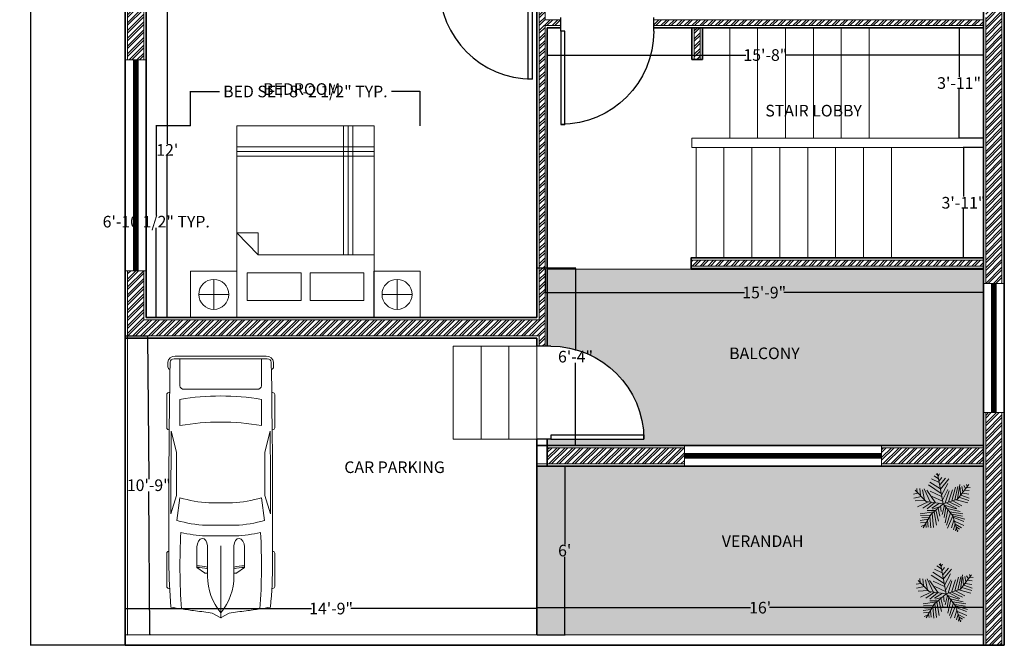
# Model space of a CAD drawing. Units: inches. Extents: x 210 to 633, y 286 to 1043.
# Tile 1 of 3: x 210 to 633, y 286 to 555. Entities that reach past the tile are written whole.
import ezdxf

# ---------------------------------------------------------------- set-up
doc = ezdxf.new("R2010")
doc.units = ezdxf.units.IN
doc.header["$MEASUREMENT"] = 0
for name, color, linetype, lineweight in [('A-ANNO-DIMS', 170, 'Continuous', 18), ('A-AREA-IDEN', 7, 'Continuous', 25), ('A-DOOR', 4, 'Continuous', 25), ('A-EQPM-VEHC', 8, 'Continuous', 18), ('A-FLOR', 7, 'Continuous', 18), ('A-FLOR-PATT', 100, 'Continuous', 13), ('A-FLOR-STRS', 7, 'Continuous', 20), ('A-GLAZ-PATT', 130, 'Continuous', 13), ('A-WALL-PATT', 35, 'Continuous', 13), ('fur', 210, 'Continuous', 18), ('L-PLNT-TREE', 100, 'Continuous', 18), ('wall', 10, 'Continuous', 35), ('wind', 130, 'Continuous', 18)]:
    doc.layers.add(name, color=color, linetype=linetype, lineweight=lineweight)
doc.styles.get("Standard").update_dxf_attribs({"font": 'arial.ttf'})
doc.dimstyles.get("Standard").update_dxf_attribs({"dimtxt": 5, "dimasz": 0.18, "dimexe": 0.18, "dimexo": 0.0625, "dimgap": 0.09, "dimtad": 0, "dimtih": 1, "dimtoh": 1, "dimdec": 0, "dimzin": 0, "dimdsep": 46, "dimlunit": 4, "dimtxsty": 'Standard', "dimcen": 0.09, "dimadec": 0, "dimazin": 0, "dimtfac": 1, "dimtdec": 0, "dimtofl": 0, "dimtmove": 0, "dimatfit": 3, "dimfxl": 1, "dimtolj": 1, "dimtzin": 0, "dimarcsym": 0})

# ---------------------------------------------------------------- blocks, each defined once
blk = doc.blocks.new('*U6')
for p, q in [((-10.186, 53.64), (-13.084, 55.962)), ((0, 0), (-10.5, 57)), ((-9.099, 51.782), (-6.563, 55.962)), ((-5.114, 28.097), (-24.676, 40.636)), ((-7.288, 39.707), (-21.778, 46.673)), ((-8.737, 47.138), (-17.069, 52.711)), ((-7.65, 43.423), (-2.578, 49.46)), ((-5.839, 35.992), (4.667, 48.067)), ((-5.114, 27.632), (10.463, 46.673)), ((-2.941, 16.486), (8.652, 37.85)), ((-47.498, 19.737), (-55.83, 18.344)), ((-31.5, 4.5), (-52.5, 25.5)), ((-48.585, 21.131), (-49.309, 29.026)), ((-43.513, 28.561), (-42.427, 15.558)), ((-38.442, 26.239), (-34.819, 7.663)), ((-35.544, 28.097), (-24.314, 3.947)), ((-14.533, 2.09), (-30.834, 25.31)), ((-3.665, 19.273), (-27.574, 35.527)), ((-24.314, 23.917), (-2.941, 13.7)), ((-1.129, 6.734), (9.014, 26.704)), ((3.942, 1.625), (11.187, 24.381)), ((10.101, 3.483), (17.708, 26.239)), ((16.259, 5.805), (23.142, 31.348)), ((22.055, 7.198), (27.489, 32.277)), ((27, 9), (48, 36)), ((27.127, 9.056), (31.112, 35.992)), ((31.836, 30.883), (32.561, 16.486)), ((35.096, 32.741), (37.27, 22.524)), ((36.183, 19.737), (48.137, 17.88)), ((38.719, 34.134), (41.979, 28.561)), ((40.53, 25.775), (48.862, 24.846)), ((43.791, 29.954), (51.036, 30.883)), ((44.153, 36.456), (45.239, 32.741)), ((-40.615, 13.7), (-55.105, 10.913)), ((-33.37, 6.269), (-52.207, 5.34)), ((-28.299, 3.483), (-47.86, -5.805)), ((-21.416, 3.018), (-38.079, -8.128)), ((0, 0), (-31.5, 4.5)), ((-15.982, 2.09), (-30.11, -9.521)), ((0, 0), (-22.5, -19.5)), ((-6.563, 1.161), (-21.416, -8.128)), ((-20.691, 13.7), (-1.129, 4.876)), ((0, 0), (27, 9)), ((0, 0), (18, -22.5)), ((6.478, 1.625), (26.04, -8.592)), ((11.187, 3.483), (30.749, -5.805)), ((18.07, 5.805), (35.096, -3.483)), ((24.229, 7.663), (46.688, 1.625)), ((29.662, 12.307), (48.137, 6.269)), ((33.285, 16.486), (48.862, 10.913)), ((-17.431, -15.094), (-42.789, -18.809)), ((-15.257, -12.772), (-30.11, -12.772)), ((-20.691, -18.345), (-17.793, -44.352)), ((-6.563, -5.805), (-19.967, -9.985)), ((-17.069, -15.094), (-12.721, -40.172)), ((-13.446, -11.378), (-8.737, -32.741)), ((-9.461, -8.592), (-6.201, -23.453)), ((-4.752, -3.483), (-3.665, -14.629)), ((2.493, -3.019), (-1.491, -20.202)), ((1.769, -2.555), (24.229, -9.521)), ((5.029, -6.27), (2.131, -25.775)), ((9.014, -11.378), (3.58, -35.992)), ((14.085, -16.951), (6.478, -40.172)), ((7.565, -9.056), (32.198, -14.629)), ((12.274, -15.094), (36.907, -18.809)), ((-28.299, -29.026), (-42.789, -31.348)), ((-24.314, -21.596), (-42.427, -22.06)), ((-30.834, -34.135), (-42.427, -35.528)), ((-26.849, -26.24), (-40.253, -25.775)), ((-22.5, -19.5), (-37.5, -45)), ((-32.646, -36.921), (-31.921, -44.352)), ((-29.023, -30.884), (-27.936, -43.887)), ((-25.038, -23.918), (-22.865, -45.281)), ((18.07, -22.524), (8.289, -45.745)), ((20.244, -30.419), (15.897, -44.816)), ((16.259, -19.738), (36.183, -22.989)), ((18, -22.5), (27, -52.5)), ((18.433, -22.524), (40.53, -29.026)), ((19.157, -25.311), (38.719, -33.206)), ((21.331, -32.741), (39.081, -40.636)), ((-34.457, -39.708), (-40.978, -42.494)), ((22.78, -37.85), (19.519, -48.532)), ((22.78, -38.314), (34.372, -44.816)), ((24.591, -45.745), (23.142, -50.854)), ((24.591, -43.423), (30.749, -47.603)), ((26.764, -49.925), (28.213, -50.854))]:
    blk.add_line(p, q)
blk = doc.blocks.new('*U8')
for p, q in [((21.1, 37.41), (21.1, 36.83)), ((46.55, 38.89), (22.35, 38.89)), ((47.8, 37.39), (47.8, 37.41)), ((87.99, 31.87), (74.76, 35.92)), ((134.31, 35.6), (119.29, 31.78)), ((135.45, 37.07), (135.45, 37.41)), ((136.7, 38.89), (160.9, 38.89)), ((162.15, 37.41), (162.15, 36.77)), ((70.03, 31.54), (86.41, 29.35)), ((138.42, 29.35), (157.25, 29.35)), ((186.47, 29.35), (167.01, 29.35)), ((186.47, -33.5), (186.47, 33.5)), ((188.4, -32.76), (188.4, 32.76)), ((164.52, 26.39), (164.52, -26.39)), ((32.27, 11.63), (36.13, 17.17)), ((36.13, 17.17), (50.94, 17.17)), ((29.77, 9.51), (51.68, 9.51)), ((32.12, 9.51), (32.12, 11.15)), ((58.92, -10.77), (58.92, 10.77)), ((66.55, -10.53), (66.55, 10.53)), ((82.74, 8.5), (82.74, -8.5)), ((186.47, -10.53), (186.47, 10.53)), ((3.27, 6.13), (0.1, 0.41)), ((0, 0), (51.68, 0)), ((0.1, -0.41), (3.27, -6.13)), ((29.77, -9.51), (51.68, -9.51)), ((32.12, -9.51), (32.12, -11.15)), ((32.27, -11.63), (36.13, -17.17)), ((36.13, -17.17), (50.94, -17.17)), ((86.41, -29.35), (70.03, -31.54)), ((87.99, -31.87), (74.76, -35.92)), ((134.31, -35.6), (119.29, -31.78)), ((157.25, -29.35), (138.42, -29.35)), ((167.01, -29.35), (186.47, -29.35)), ((21.1, -37.41), (21.1, -36.83)), ((46.55, -38.89), (22.35, -38.89)), ((47.8, -37.39), (47.8, -37.41)), ((135.45, -37.07), (135.45, -37.41)), ((136.7, -38.89), (160.9, -38.89)), ((162.15, -37.41), (162.15, -36.77))]:
    blk.add_line(p, q)
for centre, major_axis, ratio, start_param, end_param in [((266.03, -27.52), (0, 313.31), 0.842304, 1.367076, 1.39176), ((41.19, -490.86), (0, 528.23), 0.842304, 0.00281, 0.075598), ((22.35, 37.41), (0, -1.48), 0.842304, 3.141593, 4.712389), ((64.48, -10555.62), (0, 10593.03), 0.842304, -0.013397, 0.002797), ((46.55, 37.41), (0, 1.48), 0.842304, -1.570796, 0), ((64.48, -10555.62), (0, -10591.55), 0.842304, 3.133765, 3.140441), ((136.7, 37.41), (0, -1.48), 0.842304, 3.141593, 4.712389), ((160.9, 37.41), (0, 1.48), 0.842304, -1.570796, 0), ((180.63, 35.84), (0, 2.22), 0.842304, -0.013017, 1.249894), ((64.48, -10556.36), (0, 10595.31), 0.842304, -0.013397, -0.013017), ((183.98, 33.5), (0, -2.96), 0.842304, 1.570796, 3.128196), ((183.98, 32.76), (0, -5.25), 0.842304, 1.570796, 3.128196), ((37.47, -593.96), (0, -623.33), 0.842304, 3.096046, 3.200911), ((134.4, 5.39), (0, -89.78), 0.842304, 4.449482, 4.652344), ((135.29, 5.39), (0, 81.77), 0.842304, 1.245306, 1.50788), ((149.6, 2.8), (0, -79.58), 0.842304, 4.372215, 4.640744), ((95.79, -3666.35), (0, -3698.24), 0.842304, 3.134049, 3.144098), ((17.08, 0), (0, 147.02), 0.842304, 4.511394, 4.913384), ((35.91, 0), (0, 147.02), 0.842304, 4.511394, 4.913384), ((167.01, 26.39), (0, 2.96), 0.842304, 0, 1.570796), ((259.18, -27.52), (0, -305.3), 0.842304, 4.528606, 4.561838), ((-204.49, 52.4), (0, -250.96), 0.842304, 1.385369, 1.434372), ((13.04, 17.01), (0, 27.42), 0.842304, 4.435146, 4.718221), ((14.2, 17.01), (0, 27.42), 0.842304, 4.435146, 4.718221), ((50.79, 13.34), (6.34, -0.36), 0.603834, -1.395552, 1.581315), ((29.77, -46.66), (0, 56.17), 0.842304, 0, 0.590319), ((32.75, 11.15), (0, 0.74), 0.842304, 0.879714, 1.570796), ((0.62, 0), (0, -0.74), 0.842304, 4.131459, 5.293319), ((-204.49, -52.4), (0, 250.96), 0.842304, -1.434372, -1.385369), ((29.77, 46.66), (0, 56.17), 0.842304, 2.551274, 3.141593), ((32.75, -11.15), (0, -0.74), 0.842304, 4.712389, 5.403472), ((13.04, -17.01), (0, -27.42), 0.842304, 1.564964, 1.848039), ((14.2, -17.01), (0, -27.42), 0.842304, 1.564964, 1.848039), ((134.4, -5.39), (0, -89.78), 0.842304, -1.510751, -1.307889), ((135.29, -5.39), (0, -81.77), 0.842304, -1.50788, -1.245306), ((149.6, -2.8), (0, -79.58), 0.842304, -1.499151, -1.230623), ((259.18, 27.52), (0, 305.3), 0.842304, 1.721348, 1.754579), ((266.03, 27.52), (0, 313.31), 0.842304, 1.749832, 1.774517), ((37.47, 593.96), (0, -623.33), 0.842304, -0.059319, 0.045547), ((167.01, -26.39), (0, -2.96), 0.842304, 4.712389, 6.283185), ((95.79, 3666.35), (0, -3698.24), 0.842304, -0.002505, 0.007544), ((183.98, -33.5), (0, 2.96), 0.842304, 3.15499, 4.712389), ((183.98, -32.76), (0, -5.25), 0.842304, 0.013397, 1.570796), ((41.19, 490.86), (0, -528.23), 0.842304, -0.075598, -0.00281), ((22.35, -37.41), (0, 1.48), 0.842304, 1.570796, 3.141593), ((64.48, 10555.62), (0, 10593.03), 0.842304, 3.138796, 3.15499), ((46.55, -37.41), (0, -1.48), 0.842304, 0, 1.570796), ((64.48, 10555.62), (0, -10591.55), 0.842304, 0.001152, 0.007828), ((136.7, -37.41), (0, -1.48), 0.842304, -1.570796, 0), ((160.9, -37.41), (0, 1.48), 0.842304, 3.141593, 4.712389), ((180.63, -35.84), (0, -2.22), 0.842304, -1.249894, 0.013017), ((64.48, 10556.36), (0, 10595.31), 0.842304, 3.15461, 3.15499)]:
    blk.add_ellipse(centre, major_axis=major_axis, ratio=ratio, start_param=start_param, end_param=end_param)
at = {"extrusion": (0, 0, -1)}
blk.add_ellipse((50.79, -13.34), major_axis=(6.34, 0.36), ratio=0.603834, start_param=-1.395552, end_param=1.581315, dxfattribs=at)
blk = doc.blocks.new('*U2')
for p, q in [((0, 0), (0, -6)), ((40, 0), (40, -6))]:
    blk.add_line(p, q)
blk.add_lwpolyline([(0, 0), (0, 40), (1.75, 40), (1.75, 0)], close=True)
blk.add_arc((0, 0), 40, 0, 90)
blk = doc.blocks.new('*D26')
at = {"layer": 'A-ANNO-DIMS', "color": 0, "lineweight": -2, "transparency": 16777216}
for p, q in [((264.44, 571.02), (273.63, 571.02)), ((273.45, 570.84), (273.45, 501.62)), ((273.45, 427.2), (273.45, 496.42)), ((264.44, 427.02), (273.63, 427.02))]:
    blk.add_line(p, q, dxfattribs=at)
at = {"layer": 'A-ANNO-DIMS', "color": 0, "transparency": 16777216}
for points in [[(273.42, 570.84), (273.48, 570.84), (273.45, 571.02)], [(273.42, 427.2), (273.48, 427.2), (273.45, 427.02)]]:
    blk.add_solid(points, dxfattribs=at)
at = {"layer": 'Defpoints', "color": 0, "transparency": 16777216}
for p in [(264.37, 571.02), (264.37, 427.02), (273.45, 427.02)]:
    blk.add_point(p, dxfattribs=at)
at = {"layer": 'A-ANNO-DIMS', "color": 0, "transparency": 16777216, "insert": (273.45, 499.02), "char_height": 5, "attachment_point": 5}
blk.add_mtext("\\A1;12'", dxfattribs=at)
blk = doc.blocks.new('*D27')
at = {"layer": 'A-ANNO-DIMS', "color": 0, "lineweight": -2, "transparency": 16777216}
for p, q in [((255.44, 419.02), (265.16, 419.1)), ((264.98, 418.92), (265.45, 357.49)), ((265.97, 290.78), (265.5, 352.2)), ((256.44, 290.52), (266.16, 290.6))]:
    blk.add_line(p, q, dxfattribs=at)
at = {"layer": 'A-ANNO-DIMS', "color": 0, "transparency": 16777216}
for points in [[(265.01, 418.92), (264.95, 418.92), (264.98, 419.1)], [(266, 290.78), (265.94, 290.78), (265.98, 290.6)]]:
    blk.add_solid(points, dxfattribs=at)
at = {"layer": 'Defpoints', "color": 0, "transparency": 16777216}
for p in [(255.37, 419.02), (264.98, 419.1), (256.37, 290.52)]:
    blk.add_point(p, dxfattribs=at)
at = {"layer": 'A-ANNO-DIMS', "color": 0, "transparency": 16777216, "insert": (265.48, 354.85), "char_height": 5, "attachment_point": 5}
blk.add_mtext('\\A1;10\'-9"', dxfattribs=at)
blk = doc.blocks.new('*D28')
at = {"layer": 'A-ANNO-DIMS', "color": 0, "lineweight": -2, "transparency": 16777216}
for p, q in [((255.37, 290.58), (255.37, 302.01)), ((255.55, 301.83), (335.43, 301.83)), ((432.19, 301.83), (352.32, 301.83)), ((432.37, 290.58), (432.37, 302.01))]:
    blk.add_line(p, q, dxfattribs=at)
at = {"layer": 'A-ANNO-DIMS', "color": 0, "transparency": 16777216}
for points in [[(255.55, 301.86), (255.55, 301.8), (255.37, 301.83)], [(432.19, 301.86), (432.19, 301.8), (432.37, 301.83)]]:
    blk.add_solid(points, dxfattribs=at)
at = {"layer": 'Defpoints', "color": 0, "transparency": 16777216}
for p in [(432.37, 301.83), (255.37, 290.52), (432.37, 290.52)]:
    blk.add_point(p, dxfattribs=at)
at = {"layer": 'A-ANNO-DIMS', "color": 0, "transparency": 16777216, "insert": (343.87, 301.83), "char_height": 5, "attachment_point": 5}
blk.add_mtext('\\A1;14\'-9"', dxfattribs=at)
blk = doc.blocks.new('*D29')
at = {"layer": 'A-ANNO-DIMS', "color": 0, "lineweight": -2, "transparency": 16777216}
for p, q in [((432.37, 290.58), (432.37, 302.39)), ((432.55, 302.21), (524.28, 302.21)), ((624.19, 302.21), (532.47, 302.21)), ((624.37, 290.58), (624.37, 302.39))]:
    blk.add_line(p, q, dxfattribs=at)
at = {"layer": 'A-ANNO-DIMS', "color": 0, "transparency": 16777216}
for points in [[(432.55, 302.24), (432.55, 302.18), (432.37, 302.21)], [(624.19, 302.24), (624.19, 302.18), (624.37, 302.21)]]:
    blk.add_solid(points, dxfattribs=at)
at = {"layer": 'Defpoints', "color": 0, "transparency": 16777216}
for p in [(624.37, 302.21), (432.37, 290.52), (624.37, 290.52)]:
    blk.add_point(p, dxfattribs=at)
at = {"layer": 'A-ANNO-DIMS', "color": 0, "transparency": 16777216, "insert": (528.37, 302.21), "char_height": 5, "attachment_point": 5}
blk.add_mtext("\\A1;16'", dxfattribs=at)
blk = doc.blocks.new('*D30')
at = {"layer": 'A-ANNO-DIMS', "color": 0, "lineweight": -2, "transparency": 16777216}
for p, q in [((432.44, 363), (444.52, 363)), ((444.34, 362.82), (444.34, 329.4)), ((444.34, 290.7), (444.34, 324.12)), ((432.44, 290.52), (444.52, 290.52))]:
    blk.add_line(p, q, dxfattribs=at)
at = {"layer": 'A-ANNO-DIMS', "color": 0, "transparency": 16777216}
for points in [[(444.31, 362.82), (444.37, 362.82), (444.34, 363)], [(444.31, 290.7), (444.37, 290.7), (444.34, 290.52)]]:
    blk.add_solid(points, dxfattribs=at)
at = {"layer": 'Defpoints', "color": 0, "transparency": 16777216}
for p in [(432.37, 363), (444.34, 363), (432.37, 290.52)]:
    blk.add_point(p, dxfattribs=at)
at = {"layer": 'A-ANNO-DIMS', "color": 0, "transparency": 16777216, "insert": (444.34, 326.76), "char_height": 5, "attachment_point": 5}
blk.add_mtext("\\A1;6'", dxfattribs=at)
blk = doc.blocks.new('*D31')
at = {"layer": 'A-ANNO-DIMS', "color": 0, "lineweight": -2, "transparency": 16777216}
for p, q in [((432.44, 448.27), (449.18, 448.27)), ((449, 448.09), (449, 412.78)), ((449, 372.18), (449, 407.49)), ((432.44, 372), (449.18, 372))]:
    blk.add_line(p, q, dxfattribs=at)
at = {"layer": 'A-ANNO-DIMS', "color": 0, "transparency": 16777216}
for points in [[(448.97, 448.09), (449.03, 448.09), (449, 448.27)], [(448.97, 372.18), (449.03, 372.18), (449, 372)]]:
    blk.add_solid(points, dxfattribs=at)
at = {"layer": 'Defpoints', "color": 0, "transparency": 16777216}
for p in [(432.37, 448.27), (449, 448.27), (432.37, 372)]:
    blk.add_point(p, dxfattribs=at)
at = {"layer": 'A-ANNO-DIMS', "color": 0, "transparency": 16777216, "insert": (449, 410.14), "char_height": 5, "attachment_point": 5}
blk.add_mtext('\\A1;6\'-4"', dxfattribs=at)
blk = doc.blocks.new('*D32')
at = {"layer": 'A-ANNO-DIMS', "color": 0, "lineweight": -2, "transparency": 16777216}
for p, q in [((435.87, 447.69), (435.87, 437.53)), ((624.37, 447.69), (624.37, 437.53)), ((436.05, 437.71), (521.68, 437.71)), ((624.19, 437.71), (538.57, 437.71))]:
    blk.add_line(p, q, dxfattribs=at)
at = {"layer": 'A-ANNO-DIMS', "color": 0, "transparency": 16777216}
for points in [[(436.05, 437.74), (436.05, 437.68), (435.87, 437.71)], [(624.19, 437.74), (624.19, 437.68), (624.37, 437.71)]]:
    blk.add_solid(points, dxfattribs=at)
at = {"layer": 'Defpoints', "color": 0, "transparency": 16777216}
for p in [(435.87, 447.75), (624.37, 447.75), (624.37, 437.71)]:
    blk.add_point(p, dxfattribs=at)
at = {"layer": 'A-ANNO-DIMS', "color": 0, "transparency": 16777216, "insert": (530.12, 437.71), "char_height": 5, "attachment_point": 5}
blk.add_mtext('\\A1;15\'-9"', dxfattribs=at)
blk = doc.blocks.new('*D33')
at = {"layer": 'A-ANNO-DIMS', "color": 0, "lineweight": -2, "transparency": 16777216}
for p, q in [((624.31, 551.52), (613.75, 551.52)), ((613.93, 551.34), (613.93, 530.43)), ((613.93, 504.23), (613.93, 525.14)), ((624.31, 504.05), (613.75, 504.05))]:
    blk.add_line(p, q, dxfattribs=at)
at = {"layer": 'A-ANNO-DIMS', "color": 0, "transparency": 16777216}
for points in [[(613.9, 551.34), (613.96, 551.34), (613.93, 551.52)], [(613.9, 504.23), (613.96, 504.23), (613.93, 504.05)]]:
    blk.add_solid(points, dxfattribs=at)
at = {"layer": 'Defpoints', "color": 0, "transparency": 16777216}
for p in [(624.37, 551.52), (613.93, 504.05), (624.37, 504.05)]:
    blk.add_point(p, dxfattribs=at)
at = {"layer": 'A-ANNO-DIMS', "color": 0, "transparency": 16777216, "insert": (613.93, 527.79), "char_height": 5, "attachment_point": 5}
blk.add_mtext('\\A1;3\'-11"', dxfattribs=at)
blk = doc.blocks.new('*D34')
at = {"layer": 'A-ANNO-DIMS', "color": 0, "lineweight": -2, "transparency": 16777216}
for p, q in [((624.31, 500.05), (615.63, 500.05)), ((615.81, 499.87), (615.81, 478.96)), ((615.81, 452.76), (615.81, 473.67)), ((624.31, 452.58), (615.63, 452.58))]:
    blk.add_line(p, q, dxfattribs=at)
at = {"layer": 'A-ANNO-DIMS', "color": 0, "transparency": 16777216}
for points in [[(615.78, 499.87), (615.84, 499.87), (615.81, 500.05)], [(615.78, 452.76), (615.84, 452.76), (615.81, 452.58)]]:
    blk.add_solid(points, dxfattribs=at)
at = {"layer": 'Defpoints', "color": 0, "transparency": 16777216}
for p in [(615.81, 500.05), (624.37, 500.05), (624.37, 452.58)]:
    blk.add_point(p, dxfattribs=at)
at = {"layer": 'A-ANNO-DIMS', "color": 0, "transparency": 16777216, "insert": (615.81, 476.31), "char_height": 5, "attachment_point": 5}
blk.add_mtext('\\A1;3\'-11"', dxfattribs=at)
blk = doc.blocks.new('*D35')
at = {"layer": 'A-ANNO-DIMS', "color": 0, "lineweight": -2, "transparency": 16777216}
for p, q in [((436.87, 551.46), (436.87, 539.65)), ((624.37, 551.46), (624.37, 539.65)), ((437.05, 539.83), (522.18, 539.83)), ((624.19, 539.83), (539.07, 539.83))]:
    blk.add_line(p, q, dxfattribs=at)
at = {"layer": 'A-ANNO-DIMS', "color": 0, "transparency": 16777216}
for points in [[(437.05, 539.86), (437.05, 539.8), (436.87, 539.83)], [(624.19, 539.86), (624.19, 539.8), (624.37, 539.83)]]:
    blk.add_solid(points, dxfattribs=at)
at = {"layer": 'Defpoints', "color": 0, "transparency": 16777216}
for p in [(436.87, 551.52), (624.37, 551.52), (624.37, 539.83)]:
    blk.add_point(p, dxfattribs=at)
at = {"layer": 'A-ANNO-DIMS', "color": 0, "transparency": 16777216, "insert": (530.62, 539.83), "char_height": 5, "attachment_point": 5}
blk.add_mtext('\\A1;15\'-8"', dxfattribs=at)
blk = doc.blocks.new('*D36')
at = {"layer": 'A-ANNO-DIMS', "color": 0, "lineweight": -2, "transparency": 16777216}
for p, q in [((255.31, 1006.02), (214.53, 1006.02)), ((214.71, 1005.84), (214.71, 648.66)), ((214.71, 286.2), (214.71, 643.38)), ((255.31, 286.02), (214.53, 286.02))]:
    blk.add_line(p, q, dxfattribs=at)
at = {"layer": 'A-ANNO-DIMS', "color": 0, "transparency": 16777216}
for points in [[(214.68, 1005.84), (214.74, 1005.84), (214.71, 1006.02)], [(214.68, 286.2), (214.74, 286.2), (214.71, 286.02)]]:
    blk.add_solid(points, dxfattribs=at)
at = {"layer": 'Defpoints', "color": 0, "transparency": 16777216}
for p in [(214.71, 1006.02), (255.37, 1006.02), (255.37, 286.02)]:
    blk.add_point(p, dxfattribs=at)
at = {"layer": 'A-ANNO-DIMS', "color": 0, "transparency": 16777216, "insert": (214.71, 646.02), "char_height": 5, "attachment_point": 5}
blk.add_mtext("\\A1;60'", dxfattribs=at)
blk = doc.blocks.new('BED-DOUBLE-WITH-NIGHTSTANDS')
for p, q in [((-9.81, -16.35), (-9.81, -3.45)), ((68.98, -16.35), (68.98, -3.45)), ((-16.26, -9.9), (-3.36, -9.9)), ((62.53, -9.9), (75.44, -9.9)), ((0, -26.92), (49.96, -26.92)), ((9.25, -26.92), (9.25, -82.32)), ((11.25, -26.92), (11.25, -82.32)), ((13.25, -26.92), (13.25, -82.32)), ((49.96, -26.92), (49.96, -36.42)), ((59.05, -36.42), (49.96, -26.92)), ((49.96, -36.42), (59.05, -36.42)), ((0, -69.31), (59.05, -69.31)), ((0, -71.31), (59.05, -71.31)), ((0, -73.31), (59.05, -73.31))]:
    blk.add_line(p, q)
for points in [[(0, 0), (59.05, 0), (59.05, -82.32), (0, -82.32)], [(-19.74, 0), (0.13, 0), (0.13, -19.81), (-19.74, -19.81)], [(59.05, 0), (78.92, 0), (78.92, -19.81), (59.05, -19.81)], [(4.4, -7.27), (27.55, -7.27), (27.55, -19.1), (4.4, -19.1)], [(31.46, -7.27), (54.61, -7.27), (54.61, -19.1), (31.46, -19.1)]]:
    blk.add_lwpolyline(points, close=True)
for centre in [(-9.81, -9.9), (68.98, -9.9)]:
    blk.add_circle(centre, 6.45)
blk = doc.blocks.new('*D41')
at = {"layer": 'A-ANNO-DIMS', "color": 0, "lineweight": -2, "transparency": 16777216}
for p, q in [((283.5, 509.41), (283.5, 524.32)), ((283.68, 524.14), (295.87, 524.14)), ((381.98, 524.14), (369.79, 524.14)), ((382.16, 509.41), (382.16, 524.32))]:
    blk.add_line(p, q, dxfattribs=at)
at = {"layer": 'A-ANNO-DIMS', "color": 0, "transparency": 16777216}
for points in [[(283.68, 524.17), (283.68, 524.11), (283.5, 524.14)], [(381.98, 524.17), (381.98, 524.11), (382.16, 524.14)]]:
    blk.add_solid(points, dxfattribs=at)
at = {"layer": 'Defpoints', "color": 0, "transparency": 16777216}
for p in [(283.5, 524.14), (283.5, 509.34), (382.16, 509.34)]:
    blk.add_point(p, dxfattribs=at)
at = {"layer": 'A-ANNO-DIMS', "color": 0, "transparency": 16777216, "insert": (332.83, 524.14), "char_height": 5, "attachment_point": 5}
blk.add_mtext('\\A1;BED SET 8\'-2 1/2" TYP.', dxfattribs=at)
blk = doc.blocks.new('*D42')
at = {"layer": 'A-ANNO-DIMS', "color": 0, "lineweight": -2, "transparency": 16777216}
for p, q in [((283.43, 509.34), (268.52, 509.34)), ((268.7, 509.16), (268.7, 470.86)), ((268.7, 427.2), (268.7, 465.51)), ((283.43, 427.02), (268.52, 427.02))]:
    blk.add_line(p, q, dxfattribs=at)
at = {"layer": 'A-ANNO-DIMS', "color": 0, "transparency": 16777216}
for points in [[(268.67, 509.16), (268.73, 509.16), (268.7, 509.34)], [(268.67, 427.2), (268.73, 427.2), (268.7, 427.02)]]:
    blk.add_solid(points, dxfattribs=at)
at = {"layer": 'Defpoints', "color": 0, "transparency": 16777216}
for p in [(283.5, 509.34), (268.7, 427.02), (283.5, 427.02)]:
    blk.add_point(p, dxfattribs=at)
at = {"layer": 'A-ANNO-DIMS', "color": 0, "transparency": 16777216, "insert": (268.7, 468.18), "char_height": 5, "attachment_point": 5}
blk.add_mtext('\\A1;6\'-10 1/2" TYP.', dxfattribs=at)

msp = doc.modelspace()

# ---------------------------------------------------------------- hatches: boundary and pattern name
at = {"layer": 'A-FLOR-PATT'}
h = msp.add_hatch(dxfattribs=at)
h.set_pattern_fill('CROSS', color=256, scale=6.1)
h.paths.add_polyline_path([(624.37, 441.57), (624.37, 447.75), (498.66, 447.75), (436.87, 447.75), (436.87, 414.65), (438.37, 414.65, -0.401453), (478.34, 376.4), (478.37, 376.4), (478.37, 374.65), (438.37, 374.65), (436.87, 374.65), (436.87, 372), (495.79, 372), (580.59, 372), (624.37, 372), (624.37, 386.08)])
h.paths.add_polyline_path([(624.37, 363), (432.37, 363), (432.37, 290.52), (624.37, 290.52)])
h.paths.add_polyline_path([(613.51, 299.37), (613.5, 299.35), (613.52, 299.34)], flags=16)
h.paths.add_polyline_path([(608.31, 308.11), (607.13, 314.56), (607.2, 314.51), (607.15, 314.45), (608.31, 308.11), (614.5, 310.17), (615.78, 311.82), (615.77, 311.95), (615.86, 311.92), (614.53, 310.22), (614.53, 310.18), (608.31, 308.11), (608.8, 307.5), (608.9, 307.47), (608.88, 307.4), (612.41, 302.99), (612.46, 302.97), (612.45, 302.94), (608.31, 308.11), (604.39, 304.71), (604.4, 304.66), (604.32, 304.65)], flags=16)
h.paths.add_polyline_path([(612.26, 338.12), (612.25, 338.1), (612.27, 338.09)], flags=16)
h.paths.add_polyline_path([(607.06, 346.86), (605.88, 353.31), (605.95, 353.26), (605.9, 353.19), (607.06, 346.86), (613.25, 348.92), (614.53, 350.56), (614.52, 350.7), (614.61, 350.67), (613.28, 348.96), (613.28, 348.93), (607.06, 346.86), (607.55, 346.25), (607.65, 346.22), (607.63, 346.15), (611.16, 341.73), (611.21, 341.72), (611.2, 341.69), (607.06, 346.86), (603.14, 343.46), (603.15, 343.41), (603.07, 343.4)], flags=16)
at = {"layer": 'A-GLAZ-PATT'}
h = msp.add_hatch(dxfattribs=at)
h.set_pattern_fill('ANSI31', color=256)
h.paths.add_polyline_path([(580.59, 368.5), (495.79, 368.5), (495.79, 366.5), (580.59, 366.5)])
h.paths.add_polyline_path([(629.87, 441.57), (627.87, 441.57), (627.87, 386.08), (629.87, 386.08)])
h.paths.add_polyline_path([(260.87, 537.72), (258.87, 537.72), (258.87, 447.09), (260.87, 447.09)])
h.paths.add_polyline_path([(260.87, 615.48), (258.87, 615.48), (258.87, 587.48), (260.87, 587.48)])
h.paths.add_polyline_path([(260.87, 685.1), (258.87, 685.1), (258.87, 657.11), (260.87, 657.11)])
h.paths.add_polyline_path([(629.87, 691.84), (627.87, 691.84), (627.87, 663.85), (629.87, 663.85)])
h.paths.add_polyline_path([(260.87, 815.6), (258.87, 815.6), (258.87, 724.96), (260.87, 724.96)])
h.paths.add_polyline_path([(629.87, 831.37), (627.87, 831.37), (627.87, 803.38), (629.87, 803.38)])
h.paths.add_polyline_path([(629.87, 963.44), (627.87, 963.44), (627.87, 872.81), (629.87, 872.81)])
h.paths.add_polyline_path([(495.13, 1002.52), (448.67, 1002.52), (448.67, 1000.52), (495.13, 1000.52)])
h.paths.add_polyline_path([(417.29, 1002.52), (370.83, 1002.52), (370.83, 1000.52), (417.29, 1000.52)])
h.paths.add_polyline_path([(260.87, 971.49), (258.87, 971.49), (258.87, 880.85), (260.87, 880.85)])
at = {"layer": 'A-WALL-PATT'}
h = msp.add_hatch(dxfattribs=at)
h.set_pattern_fill('ANSI32', color=256, scale=6.3)
h.paths.add_polyline_path([(502.57, 551.52), (500.07, 551.52), (500.07, 537.88), (502.57, 537.88)])
h.paths.add_polyline_path([(632.37, 728.63), (627.37, 728.63, -0.012506), (625.37, 728.68), (625.37, 691.84), (632.37, 691.84)])
h = msp.add_hatch(dxfattribs=at)
h.set_pattern_fill('ANSI32', color=256, scale=6.3)
h.paths.add_polyline_path([(632.37, 663.85), (625.37, 663.85), (625.37, 556.02), (625.37, 441.57), (632.37, 441.57)])
h.paths.add_polyline_path([(632.37, 386.08), (625.37, 386.08), (625.37, 289.52), (625.37, 286.02), (632.37, 286.02), (632.37, 287.02)])
h.paths.add_polyline_path([(624.37, 371), (580.59, 371), (580.59, 364), (624.37, 364)])
h.paths.add_polyline_path([(495.79, 371), (436.87, 371), (436.87, 364), (495.79, 364)])
h = msp.add_hatch(dxfattribs=at)
h.set_pattern_fill('ANSI32', color=256, scale=6.3)
h.paths.add_polyline_path([(263.37, 587.48), (256.37, 587.48), (256.37, 537.72), (263.37, 537.72)])
h.paths.add_polyline_path([(354.65, 574.52), (264.37, 574.52), (264.37, 572.02), (354.65, 572.02)])
h = msp.add_hatch(dxfattribs=at)
h.set_pattern_fill('ANSI32', color=256, scale=6.3)
h.paths.add_polyline_path([(442.64, 555.02), (435.87, 555.02), (435.87, 552.52), (442.64, 552.52)])
h.paths.add_polyline_path([(435.87, 574.52), (433.37, 574.52), (433.37, 414.65), (435.87, 414.65)])
h.paths.add_polyline_path([(433.37, 574.52), (430.4, 574.52), (430.4, 572.02), (433.37, 572.02)])
h = msp.add_hatch(dxfattribs=at)
h.set_pattern_fill('ANSI32', color=256, scale=6.3)
h.paths.add_polyline_path([(624.37, 555.02), (482.64, 555.02), (482.64, 552.52), (624.37, 552.52)])
h = msp.add_hatch(dxfattribs=at)
h.set_pattern_fill('ANSI32', color=256, scale=6.3)
h.paths.add_polyline_path([(624.37, 451.58), (498.66, 451.58), (498.66, 449.08), (624.37, 449.08)])
h = msp.add_hatch(dxfattribs=at)
h.set_pattern_fill('ANSI32', color=256, scale=6.3)
h.paths.add_polyline_path([(433.37, 426.02), (263.37, 426.02), (263.37, 447.09), (256.37, 447.09), (256.37, 419.02), (433.37, 419.02)])

# ---------------------------------------------------------------- linework, layer by layer
at = {"layer": 'A-FLOR'}
for p, q in [((498.66, 447.75), (436.87, 447.75)), ((432.37, 290.52), (255.37, 290.52)), ((432.37, 290.52), (624.37, 290.52))]:
    msp.add_line(p, q, dxfattribs=at)
at = {"layer": 'A-FLOR-STRS'}
for p, q in [((515.28, 504.05), (515.28, 551.52)), ((527.28, 504.05), (527.28, 551.52)), ((539.28, 504.05), (539.28, 551.52)), ((551.28, 504.05), (551.28, 551.52)), ((563.28, 504.05), (563.28, 551.52)), ((575.28, 504.05), (575.28, 551.52)), ((624.37, 504.05), (499.07, 504.05)), ((499.07, 500.05), (499.07, 504.05)), ((624.37, 500.05), (499.07, 500.05)), ((500.82, 500.05), (500.82, 452.58)), ((512.82, 500.05), (512.82, 452.58)), ((524.82, 500.05), (524.82, 452.58)), ((536.82, 500.05), (536.82, 452.58)), ((548.82, 500.05), (548.82, 452.58)), ((560.82, 500.05), (560.82, 452.58)), ((572.82, 500.05), (572.82, 452.58)), ((584.82, 500.05), (584.82, 452.58)), ((396.37, 374.65), (396.37, 414.65)), ((396.37, 414.65), (432.37, 414.65)), ((408.37, 374.65), (408.37, 414.65)), ((420.37, 374.65), (420.37, 414.65)), ((432.37, 374.65), (432.37, 414.65)), ((396.37, 374.65), (432.37, 374.65))]:
    msp.add_line(p, q, dxfattribs=at)
at = {"layer": 'A-WALL-PATT'}
for p, q in [((632.37, 441.57), (632.37, 663.85)), ((256.37, 587.48), (256.37, 537.72)), ((263.37, 587.48), (263.37, 537.72)), ((433.37, 426.02), (433.37, 572.02)), ((433.37, 426.02), (433.37, 572.02)), ((435.87, 574.52), (435.87, 555.02)), ((442.64, 555.02), (435.87, 555.02)), ((435.87, 555.02), (442.64, 555.02)), ((442.64, 555.02), (442.64, 552.52)), ((624.37, 555.02), (482.64, 555.02)), ((625.37, 556.02), (625.37, 441.57)), ((435.87, 418.02), (435.87, 552.52)), ((442.64, 552.52), (435.87, 552.52)), ((442.64, 552.52), (435.87, 552.52)), ((435.87, 552.52), (435.87, 414.65)), ((624.37, 552.52), (482.64, 552.52)), ((500.07, 551.52), (500.07, 537.88)), ((502.57, 537.88), (502.57, 551.52)), ((624.37, 451.58), (498.66, 451.58)), ((624.37, 449.08), (498.66, 449.08)), ((256.37, 447.09), (256.37, 290.52)), ((256.37, 419.02), (256.37, 447.09)), ((256.37, 447.09), (263.37, 447.09)), ((263.37, 447.09), (263.37, 426.02)), ((263.37, 447.09), (263.37, 426.02)), ((263.37, 426.02), (433.37, 426.02)), ((263.37, 426.02), (433.37, 426.02)), ((264.37, 419.02), (256.37, 419.02)), ((433.37, 419.02), (256.37, 419.02)), ((264.37, 419.02), (433.37, 419.02)), ((433.37, 419.02), (433.37, 414.65)), ((433.37, 414.65), (433.37, 419.02)), ((435.87, 418.02), (435.87, 414.65)), ((625.37, 289.52), (625.37, 386.08)), ((632.37, 287.02), (632.37, 386.08)), ((495.79, 371), (436.87, 371)), ((624.37, 371), (580.59, 371)), ((495.79, 364), (432.37, 364)), ((624.37, 364), (580.59, 364)), ((625.37, 290.52), (625.37, 286.02)), ((632.37, 287.02), (632.37, 286.02))]:
    msp.add_line(p, q, dxfattribs=at)
at = {"layer": 'wall'}
for p, q in [((255.37, 1006.02), (255.37, 286.02)), ((264.37, 848.52), (264.37, 427.02)), ((624.37, 290.52), (624.37, 728.74)), ((633.37, 286.02), (633.37, 728.63)), ((624.37, 663.85), (624.37, 441.57)), ((633.37, 441.57), (633.37, 663.85)), ((255.37, 537.72), (255.37, 587.48)), ((264.37, 587.48), (264.37, 537.72)), ((264.37, 571.02), (264.37, 427.02)), ((432.37, 427.02), (432.37, 571.02)), ((432.37, 571.02), (432.37, 427.02)), ((436.87, 418.02), (436.87, 551.52)), ((436.87, 551.52), (436.87, 503.52)), ((442.64, 551.52), (436.87, 551.52)), ((436.87, 414.65), (436.87, 551.52)), ((436.87, 551.52), (442.64, 551.52)), ((624.37, 551.52), (482.64, 551.52)), ((482.64, 551.52), (624.37, 551.52)), ((499.07, 551.52), (499.07, 537.88)), ((499.07, 551.52), (499.07, 537.88)), ((503.57, 537.88), (503.57, 551.52)), ((503.57, 551.52), (503.57, 537.88)), ((624.37, 551.52), (624.37, 452.58)), ((499.07, 537.88), (503.57, 537.88)), ((624.37, 413.52), (624.37, 533.52)), ((624.37, 452.58), (498.66, 452.58)), ((498.66, 452.58), (498.66, 448.08)), ((498.66, 452.58), (498.66, 448.08)), ((624.37, 452.58), (584.82, 452.58)), ((255.37, 447.09), (255.37, 418.02)), ((264.37, 427.02), (264.37, 447.09)), ((624.37, 448.08), (498.66, 448.08)), ((264.37, 427.02), (432.37, 427.02)), ((432.37, 427.02), (264.37, 427.02)), ((255.37, 418.02), (432.37, 418.02)), ((264.37, 418.02), (256.37, 418.02)), ((264.37, 418.02), (432.37, 418.02)), ((264.37, 418.02), (432.37, 418.02)), ((432.37, 418.02), (432.37, 414.65)), ((432.37, 418.02), (432.37, 414.65)), ((436.87, 418.02), (436.87, 414.65)), ((624.37, 290.52), (624.37, 404.52)), ((624.37, 386.08), (624.37, 286.02)), ((633.37, 286.02), (633.37, 386.08)), ((432.37, 290.52), (432.37, 374.65)), ((432.37, 374.65), (432.37, 290.52)), ((436.87, 374.65), (436.87, 363)), ((432.37, 372), (495.79, 372)), ((624.37, 372), (436.87, 372)), ((580.59, 372), (624.37, 372)), ((624.37, 363), (432.37, 363)), ((432.37, 363), (495.79, 363)), ((580.59, 363), (623.75, 363)), ((623.75, 363), (624.37, 363)), ((255.37, 286.02), (633.37, 286.02))]:
    msp.add_line(p, q, dxfattribs=at)
msp.add_lwpolyline([(498.66, 447.75), (624.37, 447.75), (624.37, 452.58), (498.66, 452.58)], close=True, dxfattribs=at)
at = {"layer": 'wind'}
for p, q in [((258.87, 447.09), (258.87, 537.72)), ((260.87, 447.09), (260.87, 537.72)), ((627.87, 386.08), (627.87, 441.57)), ((629.87, 386.08), (629.87, 441.57)), ((495.79, 368.5), (580.59, 368.5)), ((495.79, 368.5), (580.59, 368.5)), ((495.79, 366.5), (580.59, 366.5))]:
    msp.add_line(p, q, dxfattribs=at)
for points in [[(264.37, 447.09), (255.37, 447.09), (255.37, 537.72), (264.37, 537.72)], [(624.37, 386.08), (633.37, 386.08), (633.37, 441.57), (624.37, 441.57)], [(495.79, 363), (580.59, 363), (580.59, 372), (495.79, 372)]]:
    msp.add_lwpolyline(points, close=True, dxfattribs=at)

# ---------------------------------------------------------------- block references
at = {"layer": 'A-DOOR', "rotation": 180}
msp.add_blockref('*U2', (430.4, 569.52), dxfattribs=at)
at = {"layer": 'A-DOOR', "xscale": -1}
for p, rotation in [((442.64, 550.02), 180), ((438.37, 374.65), 270)]:
    msp.add_blockref('*U2', p, dxfattribs=dict(at, rotation=rotation))
at = {"layer": 'A-EQPM-VEHC', "xscale": 0.5968220203240785, "yscale": 0.5968220203240785, "zscale": 0.5968220203240785, "rotation": 90}
msp.add_blockref('*U8', (296.42, 297.9), dxfattribs=at)
at = {"layer": 'fur', "rotation": 180}
msp.add_blockref('BED-DOUBLE-WITH-NIGHTSTANDS', (362.42, 427.02), dxfattribs=at)
at = {"layer": 'L-PLNT-TREE', "xscale": 0.2291041562016436, "yscale": 0.2291041562016436, "zscale": 0.2291041562016436}
for p in [(607.06, 346.86), (608.31, 308.11)]:
    msp.add_blockref('*U6', p, dxfattribs=at)

# ---------------------------------------------------------------- texts
at = {"layer": 'A-AREA-IDEN', "char_height": 5, "attachment_point": 1}
for s, insert in [('BEDROOM', (314.69, 527.7)), ('STAIR LOBBY', (530.62, 518.41)), ('BALCONY', (515.07, 414.07)), ('CAR PARKING', (349.57, 365.1)), ('VERANDAH', (511.89, 333.3))]:
    msp.add_mtext_dynamic_manual_height_columns(s, width=1430.1061, gutter_width=25, heights=[0], dxfattribs=dict(at, insert=insert))

# ---------------------------------------------------------------- dimensions: what is measured, and where the dimension line sits
at = {"layer": 'A-ANNO-DIMS'}
for base, p1, p2, picture, middle in [((214.71, 1006.02), (255.37, 286.02), (255.37, 1006.02), '*D36', (214.71, 646.02)), ((273.45, 427.02), (264.37, 571.02), (264.37, 427.02), '*D26', (273.45, 499.02)), ((613.93, 504.05), (624.37, 551.52), (624.37, 504.05), '*D33', (613.93, 527.79)), ((615.81, 500.05), (624.37, 452.58), (624.37, 500.05), '*D34', (615.81, 476.31)), ((444.34, 363), (432.37, 290.52), (432.37, 363), '*D30', (444.34, 326.76))]:
    dim = msp.add_linear_dim(base=base, p1=p1, p2=p2, angle=90, dimstyle='Standard', override={"dimclrd": 0, "dimclre": 0, "dimclrt": 0}, dxfattribs=at)
    dim.commit()
    dim.dimension.update_dxf_attribs({"geometry": picture, "text_midpoint": middle})
for base, p1, p2, picture, middle in [((624.37354481, 539.83130185), (436.87354481, 551.52178869), (624.37354481, 551.52178869), '*D35', (530.62354481, 539.83130185)), ((624.37354481, 437.70853834), (435.87354481, 447.75007533), (624.37354481, 447.75007533), '*D32', (530.12354481, 437.70853834)), ((432.37, 301.83), (255.37, 290.52), (432.37, 290.52), '*D28', (343.87, 301.83)), ((624.37, 302.21), (432.37, 290.52), (624.37, 290.52), '*D29', (528.37, 302.21))]:
    dim = msp.add_linear_dim(base=base, p1=p1, p2=p2, dimstyle='Standard', override={"dimclrd": 0, "dimclre": 0, "dimclrt": 0}, dxfattribs=at)
    dim.commit()
    dim.dimension.update_dxf_attribs({"geometry": picture, "text_midpoint": middle})
for base, p1, p2, angle, text, picture, middle in [((283.5, 524.14), (382.16, 509.34), (283.5, 509.34), 180, 'BED SET <> TYP.', '*D41', (332.83, 524.14)), ((268.7, 427.02), (283.5, 509.34), (283.5, 427.02), 270, '<> TYP.', '*D42', (268.7, 468.18))]:
    dim = msp.add_linear_dim(base=base, p1=p1, p2=p2, angle=angle, text=text, dimstyle='Standard', override={"dimdec": 1, "dimlfac": 1, "dimrnd": 0, "dimzin": 1, "dimdsep": 46, "dimlunit": 4, "dimfrac": 2}, dxfattribs=at)
    dim.commit()
    dim.dimension.update_dxf_attribs({"geometry": picture, "text_midpoint": middle})
for p1, p2, distance, picture, middle in [((432.37, 372), (432.37, 448.27), -16.62, '*D31', (449, 410.14)), ((256.37, 290.52), (255.37, 419.02), -9.6, '*D27', (265.48, 354.85))]:
    dim = msp.add_aligned_dim(p1=p1, p2=p2, distance=distance, dimstyle='Standard', override={"dimclrd": 0, "dimclre": 0, "dimclrt": 0}, dxfattribs=at)
    dim.commit()
    dim.dimension.update_dxf_attribs({"geometry": picture, "text_midpoint": middle})

doc.saveas('drawing.dxf')
